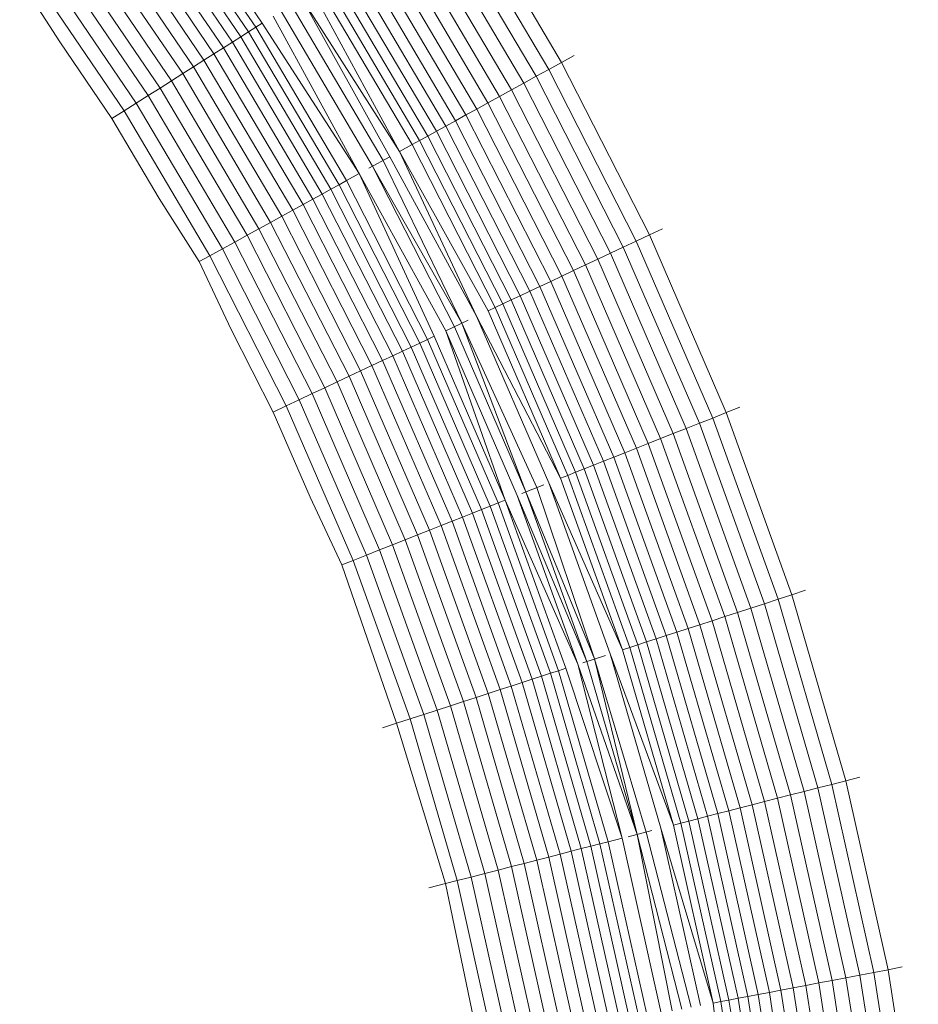
# Model space of a CAD drawing. Units: inches. Extents: x 64 to 1167, y 117 to 939.
# Tile 51 of 56: x 1130.5976 to 1130.7402, y 501.0288 to 501.185. Entities that reach past the tile are written whole.
import ezdxf

# ---------------------------------------------------------------- set-up
doc = ezdxf.new("R2010")
doc.units = ezdxf.units.IN
doc.header["$MEASUREMENT"] = 0
doc.layers.add('A-FLOR-FIXT', color=8, linetype='Continuous', lineweight=18)

msp = doc.modelspace()

# ---------------------------------------------------------------- linework, layer by layer
at = {"layer": 'A-FLOR-FIXT'}
for p, q in [((1130.63609, 501.18446), (1130.62016, 501.2079)), ((1130.63393, 501.18309), (1130.61809, 501.2064)), ((1130.63507, 501.18381), (1130.61918, 501.20719)), ((1130.63269, 501.1823), (1130.6169, 501.20554)), ((1130.68357, 501.17823), (1130.66794, 501.20467)), ((1130.62994, 501.18055), (1130.61426, 501.20362)), ((1130.63136, 501.18146), (1130.61563, 501.20461)), ((1130.68156, 501.17713), (1130.666, 501.20344)), ((1130.62843, 501.1796), (1130.61282, 501.20257)), ((1130.67956, 501.17603), (1130.66407, 501.20222)), ((1130.62519, 501.17754), (1130.60971, 501.20031)), ((1130.62684, 501.17859), (1130.6113, 501.20146)), ((1130.67759, 501.17494), (1130.66217, 501.20101)), ((1130.62347, 501.17645), (1130.60806, 501.19911)), ((1130.67376, 501.17284), (1130.65848, 501.19867)), ((1130.67565, 501.17388), (1130.66031, 501.19983)), ((1130.62169, 501.17532), (1130.60636, 501.19788)), ((1130.67191, 501.17183), (1130.65671, 501.19754)), ((1130.618, 501.17298), (1130.60283, 501.19531)), ((1130.61987, 501.17416), (1130.60461, 501.19661)), ((1130.66841, 501.1699), (1130.65333, 501.1954)), ((1130.67013, 501.17084), (1130.65499, 501.19645)), ((1130.6161, 501.17177), (1130.60101, 501.19399)), ((1130.66677, 501.16899), (1130.65175, 501.19439)), ((1130.61418, 501.17055), (1130.59916, 501.19265)), ((1130.66372, 501.16732), (1130.64881, 501.19253)), ((1130.6652, 501.16813), (1130.65024, 501.19344)), ((1130.60397, 501.18149), (1130.59761, 501.19152)), ((1130.66106, 501.16586), (1130.64624, 501.1909)), ((1130.66234, 501.16656), (1130.64748, 501.19169)), ((1130.65786, 501.1641), (1130.64408, 501.18953)), ((1130.65988, 501.16521), (1130.64511, 501.19018)), ((1130.65786, 501.1641), (1130.64236, 501.18843)), ((1130.65631, 501.16325), (1130.64236, 501.18843)), ((1130.65361, 501.16176), (1130.63907, 501.18635)), ((1130.65526, 501.16267), (1130.64066, 501.18736)), ((1130.63507, 501.18381), (1130.63609, 501.18446)), ((1130.65148, 501.16059), (1130.63609, 501.18446)), ((1130.65148, 501.16059), (1130.63782, 501.18556)), ((1130.63269, 501.1823), (1130.63393, 501.18309)), ((1130.63393, 501.18309), (1130.63507, 501.18381)), ((1130.64828, 501.15883), (1130.63393, 501.18309)), ((1130.64945, 501.15948), (1130.63507, 501.18381)), ((1130.61224, 501.16932), (1130.60397, 501.18149)), ((1130.62994, 501.18055), (1130.63136, 501.18146)), ((1130.63136, 501.18146), (1130.63269, 501.1823)), ((1130.64561, 501.15736), (1130.63136, 501.18146)), ((1130.64699, 501.15812), (1130.63269, 501.1823)), ((1130.62843, 501.1796), (1130.62994, 501.18055)), ((1130.64413, 501.15655), (1130.62994, 501.18055)), ((1130.62519, 501.17754), (1130.62684, 501.17859)), ((1130.62684, 501.17859), (1130.62843, 501.1796)), ((1130.64092, 501.15479), (1130.62684, 501.17859)), ((1130.64257, 501.15569), (1130.62843, 501.1796)), ((1130.68156, 501.17713), (1130.68357, 501.17823)), ((1130.68357, 501.17823), (1130.68559, 501.17935)), ((1130.69751, 501.15087), (1130.68357, 501.17823)), ((1130.62347, 501.17645), (1130.62519, 501.17754)), ((1130.6392, 501.15384), (1130.62519, 501.17754)), ((1130.67956, 501.17603), (1130.68156, 501.17713)), ((1130.69543, 501.14989), (1130.68156, 501.17713)), ((1130.61987, 501.17416), (1130.62169, 501.17532)), ((1130.62169, 501.17532), (1130.62347, 501.17645)), ((1130.63557, 501.15185), (1130.62169, 501.17532)), ((1130.63742, 501.15286), (1130.62347, 501.17645)), ((1130.67759, 501.17494), (1130.67956, 501.17603)), ((1130.69337, 501.14892), (1130.67956, 501.17603)), ((1130.618, 501.17298), (1130.61987, 501.17416)), ((1130.63368, 501.15081), (1130.61987, 501.17416)), ((1130.67376, 501.17284), (1130.67565, 501.17388)), ((1130.67565, 501.17388), (1130.67759, 501.17494)), ((1130.68934, 501.14702), (1130.67565, 501.17388)), ((1130.69134, 501.14796), (1130.67759, 501.17494)), ((1130.6161, 501.17177), (1130.618, 501.17298)), ((1130.63174, 501.14974), (1130.618, 501.17298)), ((1130.67191, 501.17183), (1130.67376, 501.17284)), ((1130.68738, 501.1461), (1130.67376, 501.17284)), ((1130.61224, 501.16932), (1130.61418, 501.17055)), ((1130.61418, 501.17055), (1130.6161, 501.17177)), ((1130.62778, 501.14756), (1130.61418, 501.17055)), ((1130.62977, 501.14866), (1130.6161, 501.17177)), ((1130.66841, 501.1699), (1130.67013, 501.17084)), ((1130.67013, 501.17084), (1130.67191, 501.17183)), ((1130.68364, 501.14434), (1130.67013, 501.17084)), ((1130.68548, 501.1452), (1130.67191, 501.17183)), ((1130.61973, 501.15666), (1130.61224, 501.16932)), ((1130.66677, 501.16899), (1130.6652, 501.16813)), ((1130.66677, 501.16899), (1130.66841, 501.1699)), ((1130.68016, 501.1427), (1130.66677, 501.16899)), ((1130.68186, 501.1435), (1130.66841, 501.1699)), ((1130.66372, 501.16732), (1130.66234, 501.16656)), ((1130.6652, 501.16813), (1130.66372, 501.16732)), ((1130.67702, 501.14123), (1130.66372, 501.16732)), ((1130.67855, 501.14194), (1130.6652, 501.16813)), ((1130.66106, 501.16586), (1130.65988, 501.16521)), ((1130.66234, 501.16656), (1130.66106, 501.16586)), ((1130.67427, 501.13993), (1130.66106, 501.16586)), ((1130.67559, 501.14055), (1130.66234, 501.16656)), ((1130.65988, 501.16521), (1130.65786, 501.1641)), ((1130.6701, 501.13797), (1130.65786, 501.1641)), ((1130.67195, 501.13884), (1130.65786, 501.1641)), ((1130.67305, 501.13936), (1130.65988, 501.16521)), ((1130.65631, 501.16325), (1130.65303, 501.16144)), ((1130.66774, 501.13686), (1130.65526, 501.16267)), ((1130.6701, 501.13797), (1130.65631, 501.16325)), ((1130.66658, 501.13631), (1130.65361, 501.16176)), ((1130.66774, 501.13686), (1130.65361, 501.16176)), ((1130.64945, 501.15948), (1130.64828, 501.15883)), ((1130.65148, 501.16059), (1130.64945, 501.15948)), ((1130.66229, 501.13429), (1130.64945, 501.15948)), ((1130.66524, 501.13568), (1130.65148, 501.16059)), ((1130.66339, 501.13481), (1130.65148, 501.16059)), ((1130.64699, 501.15812), (1130.64561, 501.15736)), ((1130.64828, 501.15883), (1130.64699, 501.15812)), ((1130.65974, 501.13309), (1130.64699, 501.15812)), ((1130.66107, 501.13372), (1130.64828, 501.15883)), ((1130.62609, 501.14663), (1130.61973, 501.15666)), ((1130.64413, 501.15655), (1130.64257, 501.15569)), ((1130.64561, 501.15736), (1130.64413, 501.15655)), ((1130.65679, 501.1317), (1130.64413, 501.15655)), ((1130.65832, 501.13242), (1130.64561, 501.15736)), ((1130.64092, 501.15479), (1130.6392, 501.15384)), ((1130.64257, 501.15569), (1130.64092, 501.15479)), ((1130.65348, 501.13015), (1130.64092, 501.15479)), ((1130.65518, 501.13094), (1130.64257, 501.15569)), ((1130.6392, 501.15384), (1130.63742, 501.15286)), ((1130.6517, 501.12931), (1130.6392, 501.15384)), ((1130.63557, 501.15185), (1130.63368, 501.15081)), ((1130.63742, 501.15286), (1130.63557, 501.15185)), ((1130.64796, 501.12755), (1130.63557, 501.15185)), ((1130.64986, 501.12844), (1130.63742, 501.15286)), ((1130.69751, 501.15087), (1130.6996, 501.15185)), ((1130.63368, 501.15081), (1130.63174, 501.14974)), ((1130.646, 501.12663), (1130.63368, 501.15081)), ((1130.69543, 501.14989), (1130.69751, 501.15087)), ((1130.70971, 501.12268), (1130.69751, 501.15087)), ((1130.62977, 501.14866), (1130.62778, 501.14756)), ((1130.63174, 501.14974), (1130.62977, 501.14866)), ((1130.64197, 501.12473), (1130.62977, 501.14866)), ((1130.644, 501.12569), (1130.63174, 501.14974)), ((1130.69134, 501.14796), (1130.69337, 501.14892)), ((1130.69337, 501.14892), (1130.69543, 501.14989)), ((1130.70546, 501.121), (1130.69337, 501.14892)), ((1130.70757, 501.12183), (1130.69543, 501.14989)), ((1130.62778, 501.14756), (1130.62609, 501.14663)), ((1130.6399, 501.12376), (1130.62778, 501.14756)), ((1130.68738, 501.1461), (1130.68934, 501.14702)), ((1130.68934, 501.14702), (1130.69134, 501.14796)), ((1130.70131, 501.11935), (1130.68934, 501.14702)), ((1130.70336, 501.12017), (1130.69134, 501.14796)), ((1130.63114, 501.13589), (1130.62609, 501.14663)), ((1130.68548, 501.1452), (1130.68738, 501.1461)), ((1130.6993, 501.11856), (1130.68738, 501.1461)), ((1130.68186, 501.1435), (1130.68364, 501.14434)), ((1130.68364, 501.14434), (1130.68548, 501.1452)), ((1130.69545, 501.11703), (1130.68364, 501.14434)), ((1130.69734, 501.11778), (1130.68548, 501.1452)), ((1130.67855, 501.14194), (1130.68016, 501.1427)), ((1130.68016, 501.1427), (1130.68186, 501.1435)), ((1130.69188, 501.11562), (1130.68016, 501.1427)), ((1130.69363, 501.11631), (1130.68186, 501.1435)), ((1130.67559, 501.14055), (1130.67702, 501.14123)), ((1130.67702, 501.14123), (1130.67855, 501.14194)), ((1130.68865, 501.11434), (1130.67702, 501.14123)), ((1130.69022, 501.11496), (1130.67855, 501.14194)), ((1130.67195, 501.13884), (1130.67305, 501.13936)), ((1130.67305, 501.13936), (1130.67427, 501.13993)), ((1130.68457, 501.11273), (1130.67305, 501.13936)), ((1130.67427, 501.13993), (1130.67559, 501.14055)), ((1130.68582, 501.11322), (1130.67427, 501.13993)), ((1130.68719, 501.11376), (1130.67559, 501.14055)), ((1130.68344, 501.11228), (1130.6701, 501.13797)), ((1130.68154, 501.11153), (1130.6701, 501.13797)), ((1130.68344, 501.11228), (1130.67195, 501.13884)), ((1130.66876, 501.13734), (1130.66524, 501.13568)), ((1130.67793, 501.1101), (1130.66658, 501.13631)), ((1130.67967, 501.11079), (1130.66774, 501.13686)), ((1130.67793, 501.1101), (1130.66774, 501.13686)), ((1130.63782, 501.12278), (1130.63114, 501.13589)), ((1130.66229, 501.13429), (1130.66339, 501.13481)), ((1130.67465, 501.1088), (1130.66339, 501.13481)), ((1130.67655, 501.10955), (1130.66524, 501.13568)), ((1130.67465, 501.1088), (1130.66524, 501.13568)), ((1130.65832, 501.13242), (1130.65974, 501.13309)), ((1130.65974, 501.13309), (1130.66107, 501.13372)), ((1130.6709, 501.10731), (1130.65974, 501.13309)), ((1130.66107, 501.13372), (1130.66229, 501.13429)), ((1130.67226, 501.10785), (1130.66107, 501.13372)), ((1130.67351, 501.10835), (1130.66229, 501.13429)), ((1130.65518, 501.13094), (1130.65679, 501.1317)), ((1130.65679, 501.1317), (1130.65832, 501.13242)), ((1130.66787, 501.10611), (1130.65679, 501.1317)), ((1130.66943, 501.10673), (1130.65832, 501.13242)), ((1130.6517, 501.12931), (1130.65348, 501.13015)), ((1130.65348, 501.13015), (1130.65518, 501.13094)), ((1130.66446, 501.10476), (1130.65348, 501.13015)), ((1130.66621, 501.10546), (1130.65518, 501.13094)), ((1130.64796, 501.12755), (1130.64986, 501.12844)), ((1130.64986, 501.12844), (1130.6517, 501.12931)), ((1130.66074, 501.10329), (1130.64986, 501.12844)), ((1130.66264, 501.10404), (1130.6517, 501.12931)), ((1130.644, 501.12569), (1130.646, 501.12663)), ((1130.646, 501.12663), (1130.64796, 501.12755)), ((1130.65678, 501.10172), (1130.646, 501.12663)), ((1130.65879, 501.10252), (1130.64796, 501.12755)), ((1130.64197, 501.12473), (1130.644, 501.12569)), ((1130.65472, 501.10091), (1130.644, 501.12569)), ((1130.63782, 501.12278), (1130.6399, 501.12376)), ((1130.6399, 501.12376), (1130.64197, 501.12473)), ((1130.65051, 501.09924), (1130.6399, 501.12376)), ((1130.65263, 501.10008), (1130.64197, 501.12473)), ((1130.70971, 501.12268), (1130.71186, 501.12353)), ((1130.64367, 501.10928), (1130.63782, 501.12278)), ((1130.70757, 501.12183), (1130.70971, 501.12268)), ((1130.72012, 501.09378), (1130.70971, 501.12268)), ((1130.70336, 501.12017), (1130.70546, 501.121)), ((1130.70546, 501.121), (1130.70757, 501.12183)), ((1130.71576, 501.09237), (1130.70546, 501.121)), ((1130.71793, 501.09307), (1130.70757, 501.12183)), ((1130.6993, 501.11856), (1130.70131, 501.11935)), ((1130.70131, 501.11935), (1130.70336, 501.12017)), ((1130.71152, 501.09099), (1130.70131, 501.11935)), ((1130.71362, 501.09167), (1130.70336, 501.12017)), ((1130.69545, 501.11703), (1130.69734, 501.11778)), ((1130.69734, 501.11778), (1130.6993, 501.11856)), ((1130.70746, 501.08967), (1130.69734, 501.11778)), ((1130.70947, 501.09032), (1130.6993, 501.11856)), ((1130.69188, 501.11562), (1130.69363, 501.11631)), ((1130.69363, 501.11631), (1130.69545, 501.11703)), ((1130.70366, 501.08844), (1130.69363, 501.11631)), ((1130.70553, 501.08904), (1130.69545, 501.11703)), ((1130.68719, 501.11376), (1130.68865, 501.11434)), ((1130.68865, 501.11434), (1130.69022, 501.11496)), ((1130.69858, 501.08679), (1130.68865, 501.11434)), ((1130.69022, 501.11496), (1130.69188, 501.11562)), ((1130.70018, 501.08731), (1130.69022, 501.11496)), ((1130.70188, 501.08786), (1130.69188, 501.11562)), ((1130.68344, 501.11228), (1130.68457, 501.11273)), ((1130.68457, 501.11273), (1130.68582, 501.11322)), ((1130.6944, 501.08543), (1130.68457, 501.11273)), ((1130.68582, 501.11322), (1130.68719, 501.11376)), ((1130.69568, 501.08584), (1130.68582, 501.11322)), ((1130.69707, 501.0863), (1130.68719, 501.11376)), ((1130.68079, 501.11123), (1130.6773, 501.10985)), ((1130.69324, 501.08505), (1130.68154, 501.11153)), ((1130.6913, 501.08442), (1130.68154, 501.11153)), ((1130.69324, 501.08505), (1130.68344, 501.11228)), ((1130.68619, 501.08276), (1130.67655, 501.10955)), ((1130.6876, 501.08322), (1130.67655, 501.10955)), ((1130.6876, 501.08322), (1130.67793, 501.1101)), ((1130.68882, 501.08361), (1130.67793, 501.1101)), ((1130.68882, 501.08361), (1130.67967, 501.11079)), ((1130.64872, 501.09853), (1130.64367, 501.10928)), ((1130.6709, 501.10731), (1130.67226, 501.10785)), ((1130.67226, 501.10785), (1130.67351, 501.10835)), ((1130.68181, 501.08134), (1130.67226, 501.10785)), ((1130.67351, 501.10835), (1130.67465, 501.1088)), ((1130.68309, 501.08175), (1130.67351, 501.10835)), ((1130.68425, 501.08213), (1130.67465, 501.1088)), ((1130.68619, 501.08276), (1130.67465, 501.1088)), ((1130.66787, 501.10611), (1130.66943, 501.10673)), ((1130.66943, 501.10673), (1130.6709, 501.10731)), ((1130.67891, 501.0804), (1130.66943, 501.10673)), ((1130.68042, 501.08088), (1130.6709, 501.10731)), ((1130.66264, 501.10404), (1130.66446, 501.10476)), ((1130.66446, 501.10476), (1130.66621, 501.10546)), ((1130.67383, 501.07874), (1130.66446, 501.10476)), ((1130.66621, 501.10546), (1130.66787, 501.10611)), ((1130.67561, 501.07932), (1130.66621, 501.10546)), ((1130.67731, 501.07988), (1130.66787, 501.10611)), ((1130.65879, 501.10252), (1130.66074, 501.10329)), ((1130.66074, 501.10329), (1130.66264, 501.10404)), ((1130.67003, 501.07751), (1130.66074, 501.10329)), ((1130.67196, 501.07814), (1130.66264, 501.10404)), ((1130.65472, 501.10091), (1130.65678, 501.10172)), ((1130.65678, 501.10172), (1130.65879, 501.10252)), ((1130.66597, 501.07619), (1130.65678, 501.10172)), ((1130.66803, 501.07686), (1130.65879, 501.10252)), ((1130.65051, 501.09924), (1130.65263, 501.10008)), ((1130.65263, 501.10008), (1130.65472, 501.10091)), ((1130.66173, 501.07481), (1130.65263, 501.10008)), ((1130.66387, 501.07551), (1130.65472, 501.10091)), ((1130.64872, 501.09853), (1130.65051, 501.09924)), ((1130.65738, 501.0734), (1130.64872, 501.09853)), ((1130.65956, 501.07411), (1130.65051, 501.09924)), ((1130.71793, 501.09307), (1130.72012, 501.09378)), ((1130.72012, 501.09378), (1130.72231, 501.0945)), ((1130.72868, 501.06429), (1130.72012, 501.09378)), ((1130.71362, 501.09167), (1130.71576, 501.09237)), ((1130.71576, 501.09237), (1130.71793, 501.09307)), ((1130.72425, 501.06315), (1130.71576, 501.09237)), ((1130.72646, 501.06372), (1130.71793, 501.09307)), ((1130.70947, 501.09032), (1130.71152, 501.09099)), ((1130.71152, 501.09099), (1130.71362, 501.09167)), ((1130.71993, 501.06204), (1130.71152, 501.09099)), ((1130.72207, 501.06259), (1130.71362, 501.09167)), ((1130.70553, 501.08904), (1130.70746, 501.08967)), ((1130.70746, 501.08967), (1130.70947, 501.09032)), ((1130.7158, 501.06098), (1130.70746, 501.08967)), ((1130.71784, 501.06151), (1130.70947, 501.09032)), ((1130.70018, 501.08731), (1130.70188, 501.08786)), ((1130.70188, 501.08786), (1130.70366, 501.08844)), ((1130.71011, 501.05952), (1130.70188, 501.08786)), ((1130.70366, 501.08844), (1130.70553, 501.08904)), ((1130.71193, 501.05999), (1130.70366, 501.08844)), ((1130.71383, 501.06048), (1130.70553, 501.08904)), ((1130.69568, 501.08584), (1130.69707, 501.0863)), ((1130.69707, 501.0863), (1130.69858, 501.08679)), ((1130.70522, 501.05827), (1130.69707, 501.0863)), ((1130.69858, 501.08679), (1130.70018, 501.08731)), ((1130.70675, 501.05866), (1130.69858, 501.08679)), ((1130.70838, 501.05908), (1130.70018, 501.08731)), ((1130.70132, 501.05726), (1130.6913, 501.08442)), ((1130.69934, 501.05676), (1130.6913, 501.08442)), ((1130.69324, 501.08505), (1130.6944, 501.08543)), ((1130.70132, 501.05726), (1130.69324, 501.08505)), ((1130.6944, 501.08543), (1130.69568, 501.08584)), ((1130.7025, 501.05757), (1130.6944, 501.08543)), ((1130.7038, 501.0579), (1130.69568, 501.08584)), ((1130.69053, 501.08417), (1130.68696, 501.08301)), ((1130.69557, 501.05579), (1130.6876, 501.08322)), ((1130.69703, 501.05616), (1130.68882, 501.08361)), ((1130.69557, 501.05579), (1130.68882, 501.08361)), ((1130.68042, 501.08088), (1130.68181, 501.08134)), ((1130.68181, 501.08134), (1130.68309, 501.08175)), ((1130.68967, 501.05427), (1130.68181, 501.08134)), ((1130.68309, 501.08175), (1130.68425, 501.08213)), ((1130.69098, 501.05461), (1130.68309, 501.08175)), ((1130.69321, 501.05518), (1130.68425, 501.08213)), ((1130.69321, 501.05518), (1130.68619, 501.08276)), ((1130.69557, 501.05579), (1130.68619, 501.08276)), ((1130.67561, 501.07932), (1130.67731, 501.07988)), ((1130.67731, 501.07988), (1130.67891, 501.0804)), ((1130.68509, 501.0531), (1130.67731, 501.07988)), ((1130.67891, 501.0804), (1130.68042, 501.08088)), ((1130.68672, 501.05352), (1130.67891, 501.0804)), ((1130.68825, 501.05391), (1130.68042, 501.08088)), ((1130.67196, 501.07814), (1130.67383, 501.07874)), ((1130.67383, 501.07874), (1130.67561, 501.07932)), ((1130.68154, 501.05219), (1130.67383, 501.07874)), ((1130.68336, 501.05265), (1130.67561, 501.07932)), ((1130.66597, 501.07619), (1130.66803, 501.07686)), ((1130.66803, 501.07686), (1130.67003, 501.07751)), ((1130.67563, 501.05067), (1130.66803, 501.07686)), ((1130.67003, 501.07751), (1130.67196, 501.07814)), ((1130.67767, 501.05119), (1130.67003, 501.07751)), ((1130.67964, 501.0517), (1130.67196, 501.07814)), ((1130.66173, 501.07481), (1130.66387, 501.07551)), ((1130.66387, 501.07551), (1130.66597, 501.07619)), ((1130.6714, 501.04958), (1130.66387, 501.07551)), ((1130.67354, 501.05013), (1130.66597, 501.07619)), ((1130.65738, 501.0734), (1130.65956, 501.07411)), ((1130.65956, 501.07411), (1130.66173, 501.07481)), ((1130.66701, 501.04846), (1130.65956, 501.07411)), ((1130.66922, 501.04902), (1130.66173, 501.07481)), ((1130.65518, 501.07269), (1130.65738, 501.0734)), ((1130.66515, 501.04798), (1130.65738, 501.0734)), ((1130.72646, 501.06372), (1130.72868, 501.06429)), ((1130.72868, 501.06429), (1130.73092, 501.06486)), ((1130.73538, 501.03432), (1130.72868, 501.06429)), ((1130.71993, 501.06204), (1130.72207, 501.06259)), ((1130.72207, 501.06259), (1130.72425, 501.06315)), ((1130.72868, 501.03304), (1130.72207, 501.06259)), ((1130.72425, 501.06315), (1130.72646, 501.06372)), ((1130.73089, 501.03346), (1130.72425, 501.06315)), ((1130.73313, 501.03389), (1130.72646, 501.06372)), ((1130.71383, 501.06048), (1130.7158, 501.06098)), ((1130.7158, 501.06098), (1130.71784, 501.06151)), ((1130.72232, 501.03182), (1130.7158, 501.06098)), ((1130.71784, 501.06151), (1130.71993, 501.06204)), ((1130.72438, 501.03222), (1130.71784, 501.06151)), ((1130.72651, 501.03262), (1130.71993, 501.06204)), ((1130.70838, 501.05908), (1130.71011, 501.05952)), ((1130.71011, 501.05952), (1130.71193, 501.05999)), ((1130.71655, 501.03072), (1130.71011, 501.05952)), ((1130.71193, 501.05999), (1130.71383, 501.06048)), ((1130.71839, 501.03108), (1130.71193, 501.05999)), ((1130.72032, 501.03144), (1130.71383, 501.06048)), ((1130.7025, 501.05757), (1130.7038, 501.0579)), ((1130.7038, 501.0579), (1130.70522, 501.05827)), ((1130.71015, 501.0295), (1130.7038, 501.0579)), ((1130.70522, 501.05827), (1130.70675, 501.05866)), ((1130.71159, 501.02978), (1130.70522, 501.05827)), ((1130.70675, 501.05866), (1130.70838, 501.05908)), ((1130.71314, 501.03007), (1130.70675, 501.05866)), ((1130.71479, 501.03039), (1130.70838, 501.05908)), ((1130.6979, 501.05639), (1130.69413, 501.05542)), ((1130.70763, 501.02902), (1130.69934, 501.05676)), ((1130.70562, 501.02864), (1130.69934, 501.05676)), ((1130.70132, 501.05726), (1130.7025, 501.05757)), ((1130.70763, 501.02902), (1130.70132, 501.05726)), ((1130.70883, 501.02925), (1130.7025, 501.05757)), ((1130.69098, 501.05461), (1130.69321, 501.05518)), ((1130.69941, 501.02745), (1130.69321, 501.05518)), ((1130.70114, 501.02779), (1130.69557, 501.05579)), ((1130.70269, 501.02808), (1130.69557, 501.05579)), ((1130.70417, 501.02836), (1130.69703, 501.05616)), ((1130.68509, 501.0531), (1130.68672, 501.05352)), ((1130.68672, 501.05352), (1130.68825, 501.05391)), ((1130.69283, 501.0262), (1130.68672, 501.05352)), ((1130.68825, 501.05391), (1130.68967, 501.05427)), ((1130.69438, 501.0265), (1130.68825, 501.05391)), ((1130.68967, 501.05427), (1130.69098, 501.05461)), ((1130.69582, 501.02677), (1130.68967, 501.05427)), ((1130.69714, 501.02702), (1130.69098, 501.05461)), ((1130.67767, 501.05119), (1130.67964, 501.0517)), ((1130.67964, 501.0517), (1130.68154, 501.05219)), ((1130.68565, 501.02483), (1130.67964, 501.0517)), ((1130.68154, 501.05219), (1130.68336, 501.05265)), ((1130.68758, 501.0252), (1130.68154, 501.05219)), ((1130.68336, 501.05265), (1130.68509, 501.0531)), ((1130.68942, 501.02555), (1130.68336, 501.05265)), ((1130.69117, 501.02588), (1130.68509, 501.0531)), ((1130.6714, 501.04958), (1130.67354, 501.05013)), ((1130.67354, 501.05013), (1130.67563, 501.05067)), ((1130.67946, 501.02365), (1130.67354, 501.05013)), ((1130.67563, 501.05067), (1130.67767, 501.05119)), ((1130.68158, 501.02405), (1130.67563, 501.05067)), ((1130.68365, 501.02445), (1130.67767, 501.05119)), ((1130.66701, 501.04846), (1130.66922, 501.04902)), ((1130.66922, 501.04902), (1130.6714, 501.04958)), ((1130.67508, 501.02281), (1130.66922, 501.04902)), ((1130.67729, 501.02323), (1130.6714, 501.04958)), ((1130.66255, 501.04731), (1130.66515, 501.04798)), ((1130.66515, 501.04798), (1130.66701, 501.04846)), ((1130.67058, 501.02196), (1130.66515, 501.04798)), ((1130.67284, 501.02239), (1130.66701, 501.04846)), ((1130.73765, 501.03475), (1130.73538, 501.03432)), ((1130.72868, 501.03304), (1130.72651, 501.03262)), ((1130.73089, 501.03346), (1130.72868, 501.03304)), ((1130.73342, 501.00313), (1130.72868, 501.03304)), ((1130.73313, 501.03389), (1130.73089, 501.03346)), ((1130.73565, 501.00341), (1130.73089, 501.03346)), ((1130.73538, 501.03432), (1130.73313, 501.03389)), ((1130.73791, 501.00369), (1130.73313, 501.03389)), ((1130.74019, 501.00398), (1130.73538, 501.03432)), ((1130.72032, 501.03144), (1130.71839, 501.03108)), ((1130.72232, 501.03182), (1130.72032, 501.03144)), ((1130.72497, 501.00206), (1130.72032, 501.03144)), ((1130.72438, 501.03222), (1130.72232, 501.03182)), ((1130.72699, 501.00232), (1130.72232, 501.03182)), ((1130.72651, 501.03262), (1130.72438, 501.03222)), ((1130.72908, 501.00258), (1130.72438, 501.03222)), ((1130.73122, 501.00285), (1130.72651, 501.03262)), ((1130.71159, 501.02978), (1130.71015, 501.0295)), ((1130.71314, 501.03007), (1130.71159, 501.02978)), ((1130.71615, 501.00095), (1130.71159, 501.02978)), ((1130.71479, 501.03039), (1130.71314, 501.03007)), ((1130.71772, 501.00114), (1130.71314, 501.03007)), ((1130.71655, 501.03072), (1130.71479, 501.03039)), ((1130.71939, 501.00135), (1130.71479, 501.03039)), ((1130.71839, 501.03108), (1130.71655, 501.03072)), ((1130.72116, 501.00158), (1130.71655, 501.03072)), ((1130.72303, 501.00181), (1130.71839, 501.03108)), ((1130.70883, 501.02925), (1130.70763, 501.02902)), ((1130.71108, 501.0003), (1130.70763, 501.02902)), ((1130.71015, 501.0295), (1130.70883, 501.02925)), ((1130.71337, 501.00059), (1130.70883, 501.02925)), ((1130.7147, 501.00076), (1130.71015, 501.0295))]:
    msp.add_line(p, q, dxfattribs=at)

doc.saveas('drawing.dxf')
